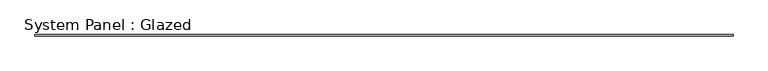
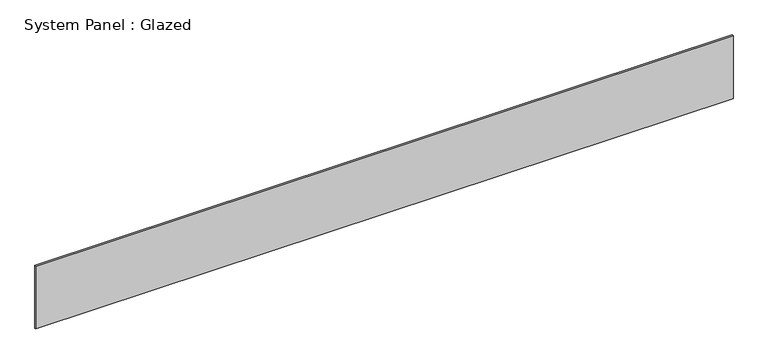
"""IFC4 building model written with IfcOpenShell, lengths in millimetres: plate geometry, System Panel : Glazed."""

from ifc_helpers import new_model, si_unit, origin, origin_with_axes, place, context, project, spatial, polyline, outline, extrude, source, transform, mapped, element, save


def system_panel_glazed_cf6986e1(model_context):
    return source(origin(), model_context, "Body", "SweptSolid", [
        extrude(outline(polyline([(6401.9831637, 19.05), (-6401.9831637, 19.05), (-6401.9831637, 44.45), (6401.9831637, 44.45), (6401.9831637, 19.05)])), origin_with_axes(), (0.0, 0.0, 1.0), 1219.2),
    ])


if __name__ == "__main__":
    model = new_model("IFC4")
    model_context = context("Model", 3, world=origin())
    ifc_project = project(units=[si_unit("LENGTHUNIT", "METRE", prefix="MILLI")], contexts=[model_context])
    site = spatial("IfcSite", under=ifc_project)
    building = spatial("IfcBuilding", under=site)
    placement = place(None, origin())
    system_panel_glazed_shape = system_panel_glazed_cf6986e1(model_context)
    element("IfcPlate", 1, ObjectType="System Panel : Glazed", at=placement, inside=building, context=model_context, shape_type="MappedRepresentation", body=[
        mapped(system_panel_glazed_shape, transform((0.0, 0.0, 0.0), x_axis=(1.0, 0.0, 0.0), y_axis=(0.0, 1.0, 0.0), z_axis=(0.0, 0.0, 1.0))),
    ])
    save(model, "model.ifc")

# Revit data of these elements
# Type "System Panel : Glazed"
#   Construction Type Id = "GSP4R"
#   Analytic Construction = "1/8 in Pilkington single glazing"
#   Visual Light Transmittance = 0.9
#   Solar Heat Gain Coefficient = 0.86
#   Heat Transfer Coefficient (U) = 1.18115 BTU/(h·ft²·°F)
# Element 1 (IfcPlate, "System Panel : Glazed")
#   Materials on its faces: "Glass"
# Materials
#   "Glass": class "Glass", colour RGB 0 128 192, transparency 0.75, Description = "Soda Lime Glass", Cost = 0
